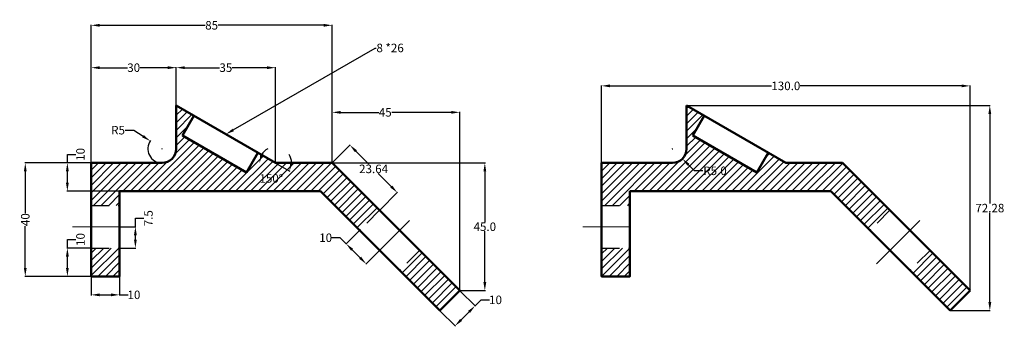
# Model space of a CAD drawing. Units: millimetres. Extents: x -10 to 337, y -40 to 68.
import ezdxf
from ezdxf import colors
from ezdxf.entities.mleader import LeaderData, LeaderLine
from ezdxf.math import Vec2, Vec3

# ---------------------------------------------------------------- set-up
doc = ezdxf.new("R2010")
doc.units = ezdxf.units.MM
doc.header["$MEASUREMENT"] = 0
doc.linetypes.add('CENTER', pattern=[50.8, 31.75, -6.35, 6.35, -6.35])
doc.linetypes.add('HIDDEN', pattern=[9.525, 6.35, -3.175])
for name, color, linetype, lineweight in [('M-CNTR', 1, 'CENTER', 18), ('M-DIMS', 3, 'Continuous', 25), ('M-HATC', 8, 'Continuous', 18), ('M-HIDN', 8, 'HIDDEN', 25), ('M-OUTL', 7, 'Continuous', 50)]:
    doc.layers.add(name, color=color, linetype=linetype, lineweight=lineweight)
doc.styles.get("Standard").update_dxf_attribs({"font": 'arial.ttf'})
doc.dimstyles.get("Standard").update_dxf_attribs({"dimtxt": 3, "dimasz": 3, "dimexe": 0.18, "dimexo": 0.0625, "dimgap": 0.09, "dimtad": 0, "dimtih": 1, "dimtoh": 1, "dimdec": 1, "dimdsep": 46, "dimtxsty": 'Standard', "dimcen": 0.09, "dimadec": 0, "dimazin": 0, "dimtfac": 1, "dimtdec": 1, "dimtofl": 0, "dimtmove": 0, "dimatfit": 3, "dimfxl": 1, "dimtolj": 1, "dimtzin": 0, "dimarcsym": 0})

# ---------------------------------------------------------------- blocks, each defined once
blk = doc.blocks.new('*D1')
at = {"layer": 'Defpoints', "color": 0, "transparency": 16777216}
for p in [(144.86, -27.53), (137.79, -34.6), (150.26, -32.93)]:
    blk.add_point(p, dxfattribs=at)
at = {"layer": 'M-DIMS', "color": 0, "lineweight": -2, "transparency": 16777216}
for p, q in [((144.9, -27.57), (150.39, -33.06)), ((150.26, -32.93), (152.39, -30.81)), ((152.39, -30.81), (155.39, -30.81)), ((137.83, -34.64), (143.32, -40.13)), ((145.32, -37.88), (148.14, -35.06))]:
    blk.add_line(p, q, dxfattribs=at)
at = {"layer": 'M-DIMS', "color": 0, "transparency": 16777216}
for points in [[(147.79, -34.7), (148.5, -35.41), (150.26, -32.93)], [(144.96, -37.53), (145.67, -38.24), (143.19, -40)]]:
    blk.add_solid(points, dxfattribs=at)
at = {"layer": 'M-DIMS', "color": 0, "transparency": 16777216, "insert": (157.48, -30.81), "char_height": 3, "attachment_point": 5}
blk.add_mtext('\\A1;10', dxfattribs=at)
blk = doc.blocks.new('*D2')
at = {"layer": 'Defpoints', "color": 0, "transparency": 16777216}
for p in [(144.86, 35.3), (99.86, 17.47), (144.86, -27.53)]:
    blk.add_point(p, dxfattribs=at)
at = {"layer": 'M-DIMS', "color": 0, "lineweight": -2, "transparency": 16777216}
for p, q in [((99.86, 17.53), (99.86, 35.48)), ((102.86, 35.3), (116.27, 35.3)), ((141.86, 35.3), (120.89, 35.3)), ((144.86, -27.47), (144.86, 35.48))]:
    blk.add_line(p, q, dxfattribs=at)
at = {"layer": 'M-DIMS', "color": 0, "transparency": 16777216}
for points in [[(102.86, 35.8), (102.86, 34.8), (99.86, 35.3)], [(141.86, 35.8), (141.86, 34.8), (144.86, 35.3)]]:
    blk.add_solid(points, dxfattribs=at)
at = {"layer": 'M-DIMS', "color": 0, "transparency": 16777216, "insert": (118.58, 35.3), "char_height": 3, "attachment_point": 5}
blk.add_mtext('\\A1;45', dxfattribs=at)
blk = doc.blocks.new('*D3')
at = {"layer": 'Defpoints', "color": 0, "transparency": 16777216}
for p in [(29.39, 46.61), (14.86, 17.47), (79.86, 17.47), (99.86, 17.47), (76.21, 13.13)]:
    blk.add_point(p, dxfattribs=at)
at = {"layer": 'M-DIMS', "color": 0, "lineweight": -2, "transparency": 16777216}
blk.add_line((79.91, 17.44), (84.93, 14.55), dxfattribs=at)
for start, end in [(118.6551, 149.3276), (0.6724, 31.3449)]:
    blk.add_arc((79.86, 17.47), 5.67, start, end, dxfattribs=at)
at = {"layer": 'M-DIMS', "color": 0, "transparency": 16777216}
for points in [[(75.46, 20.23), (74.5, 20.5), (74.19, 17.47)], [(86.01, 17.41), (85.05, 17.67), (84.77, 14.64)]]:
    blk.add_solid(points, dxfattribs=at)
at = {"layer": 'M-DIMS', "color": 0, "transparency": 16777216, "insert": (78.39, 11.99), "char_height": 3, "attachment_point": 5}
blk.add_mtext('\\A1;150°', dxfattribs=at)
blk = doc.blocks.new('*D4')
at = {"layer": 'Defpoints', "color": 0, "transparency": 16777216}
for p in [(109.5, -6.31), (104.78, -11.03), (116.57, -13.39)]:
    blk.add_point(p, dxfattribs=at)
at = {"layer": 'M-DIMS', "color": 0, "lineweight": -2, "transparency": 16777216}
for p, q in [((109.46, -6.36), (104.66, -11.16)), ((102.66, -8.91), (99.66, -8.91)), ((104.78, -11.03), (102.66, -8.91)), ((109.73, -15.98), (106.9, -13.16)), ((116.53, -13.43), (111.73, -18.23))]:
    blk.add_line(p, q, dxfattribs=at)
at = {"layer": 'M-DIMS', "color": 0, "transparency": 16777216}
for points in [[(107.26, -12.8), (106.55, -13.51), (104.78, -11.03)], [(110.09, -15.63), (109.38, -16.34), (111.85, -18.11)]]:
    blk.add_solid(points, dxfattribs=at)
at = {"layer": 'M-DIMS', "color": 0, "transparency": 16777216, "insert": (97.57, -8.91), "char_height": 3, "attachment_point": 5}
blk.add_mtext('\\A1;10', dxfattribs=at)
blk = doc.blocks.new('*D5')
at = {"layer": 'Defpoints', "color": 0, "transparency": 16777216}
for p in [(99.86, 65.99), (14.86, 17.47), (99.86, 17.47)]:
    blk.add_point(p, dxfattribs=at)
at = {"layer": 'M-DIMS', "color": 0, "lineweight": -2, "transparency": 16777216}
for p, q in [((14.86, 17.53), (14.86, 66.17)), ((17.86, 65.99), (55.11, 65.99)), ((96.86, 65.99), (59.61, 65.99)), ((99.86, 17.53), (99.86, 66.17))]:
    blk.add_line(p, q, dxfattribs=at)
at = {"layer": 'M-DIMS', "color": 0, "transparency": 16777216}
for points in [[(17.86, 66.49), (17.86, 65.49), (14.86, 65.99)], [(96.86, 66.49), (96.86, 65.49), (99.86, 65.99)]]:
    blk.add_solid(points, dxfattribs=at)
at = {"layer": 'M-DIMS', "color": 0, "transparency": 16777216, "insert": (57.36, 65.99), "char_height": 3, "attachment_point": 5}
blk.add_mtext('\\A1;85', dxfattribs=at)
blk = doc.blocks.new('*D6')
at = {"layer": 'Defpoints', "color": 0, "transparency": 16777216}
for p in [(44.86, 51.05), (44.86, 37.68), (14.86, 17.47)]:
    blk.add_point(p, dxfattribs=at)
at = {"layer": 'M-DIMS', "color": 0, "lineweight": -2, "transparency": 16777216}
for p, q in [((14.86, 17.53), (14.86, 51.23)), ((17.86, 51.05), (27.63, 51.05)), ((41.86, 51.05), (32.09, 51.05)), ((44.86, 37.74), (44.86, 51.23))]:
    blk.add_line(p, q, dxfattribs=at)
at = {"layer": 'M-DIMS', "color": 0, "transparency": 16777216}
for points in [[(17.86, 51.55), (17.86, 50.55), (14.86, 51.05)], [(41.86, 51.55), (41.86, 50.55), (44.86, 51.05)]]:
    blk.add_solid(points, dxfattribs=at)
at = {"layer": 'M-DIMS', "color": 0, "transparency": 16777216, "insert": (29.86, 51.05), "char_height": 3, "attachment_point": 5}
blk.add_mtext('\\A1;30', dxfattribs=at)
blk = doc.blocks.new('*D7')
at = {"layer": 'Defpoints', "color": 0, "transparency": 16777216}
for p in [(79.86, 51.05), (44.86, 37.68), (79.86, 17.47)]:
    blk.add_point(p, dxfattribs=at)
at = {"layer": 'M-DIMS', "color": 0, "lineweight": -2, "transparency": 16777216}
for p, q in [((44.86, 37.74), (44.86, 51.23)), ((47.86, 51.05), (60.11, 51.05)), ((76.86, 51.05), (64.61, 51.05)), ((79.86, 17.53), (79.86, 51.23))]:
    blk.add_line(p, q, dxfattribs=at)
at = {"layer": 'M-DIMS', "color": 0, "transparency": 16777216}
for points in [[(47.86, 51.55), (47.86, 50.55), (44.86, 51.05)], [(76.86, 51.55), (76.86, 50.55), (79.86, 51.05)]]:
    blk.add_solid(points, dxfattribs=at)
at = {"layer": 'M-DIMS', "color": 0, "transparency": 16777216, "insert": (62.36, 51.05), "char_height": 3, "attachment_point": 5}
blk.add_mtext('\\A1;35', dxfattribs=at)
blk = doc.blocks.new('*D8')
at = {"layer": 'Defpoints', "color": 0, "transparency": 16777216}
for p in [(35.68, 25.21), (39.86, 22.47)]:
    blk.add_point(p, dxfattribs=at)
at = {"layer": 'M-DIMS', "color": 0, "lineweight": -2, "transparency": 16777216}
for p, q in [((26.86, 29.02), (29.86, 29.02)), ((29.86, 29.02), (33.17, 26.86)), ((39.77, 22.47), (39.95, 22.47)), ((39.86, 22.38), (39.86, 22.56))]:
    blk.add_line(p, q, dxfattribs=at)
blk.add_arc((39.86, 22.47), 5, 144.7166, 269.2838, dxfattribs=at)
at = {"layer": 'M-DIMS', "color": 0, "transparency": 16777216}
blk.add_solid([(33.44, 27.27), (32.89, 26.44), (35.68, 25.21)], dxfattribs=at)
at = {"layer": 'M-DIMS', "color": 0, "transparency": 16777216, "insert": (24.34, 29.02), "char_height": 3, "attachment_point": 5}
blk.add_mtext('\\A1;R5', dxfattribs=at)
blk = doc.blocks.new('*D9')
at = {"layer": 'Defpoints', "color": 0, "transparency": 16777216}
for p in [(14.86, -22.53), (24.86, -22.53), (24.86, -29.04)]:
    blk.add_point(p, dxfattribs=at)
at = {"layer": 'M-DIMS', "color": 0, "lineweight": -2, "transparency": 16777216}
for p, q in [((14.86, -22.59), (14.86, -29.22)), ((24.86, -22.59), (24.86, -29.22)), ((17.86, -29.04), (21.86, -29.04)), ((24.86, -29.04), (27.86, -29.04))]:
    blk.add_line(p, q, dxfattribs=at)
at = {"layer": 'M-DIMS', "color": 0, "transparency": 16777216}
for points in [[(17.86, -28.54), (17.86, -29.54), (14.86, -29.04)], [(21.86, -28.54), (21.86, -29.54), (24.86, -29.04)]]:
    blk.add_solid(points, dxfattribs=at)
at = {"layer": 'M-DIMS', "color": 0, "transparency": 16777216, "insert": (29.95, -29.04), "char_height": 3, "attachment_point": 5}
blk.add_mtext('\\A1;10', dxfattribs=at)
blk = doc.blocks.new('*D10')
at = {"layer": 'Defpoints', "color": 0, "transparency": 16777216}
for p in [(6.47, -12.53), (14.86, -12.53), (14.86, -22.53)]:
    blk.add_point(p, dxfattribs=at)
at = {"layer": 'M-DIMS', "color": 0, "lineweight": -2, "transparency": 16777216}
for p, q in [((6.47, -12.53), (6.47, -9.53)), ((6.47, -9.53), (9.47, -9.53)), ((14.8, -12.53), (6.29, -12.53)), ((6.47, -19.53), (6.47, -15.53)), ((14.8, -22.53), (6.29, -22.53))]:
    blk.add_line(p, q, dxfattribs=at)
at = {"layer": 'M-DIMS', "color": 0, "transparency": 16777216}
for points in [[(5.97, -15.53), (6.97, -15.53), (6.47, -12.53)], [(5.97, -19.53), (6.97, -19.53), (6.47, -22.53)]]:
    blk.add_solid(points, dxfattribs=at)
at = {"layer": 'M-DIMS', "color": 0, "transparency": 16777216, "insert": (11.09, -9.53), "char_height": 3, "attachment_point": 5, "rotation": 90}
blk.add_mtext('\\A1;10', dxfattribs=at)
blk = doc.blocks.new('*D11')
at = {"layer": 'Defpoints', "color": 0, "transparency": 16777216}
for p in [(24.86, -5.03), (30.45, -5.03), (24.86, -12.53)]:
    blk.add_point(p, dxfattribs=at)
at = {"layer": 'M-DIMS', "color": 0, "lineweight": -2, "transparency": 16777216}
for p, q in [((30.45, -5.03), (30.45, -2.03)), ((30.45, -2.03), (33.45, -2.03)), ((24.92, -5.03), (30.63, -5.03)), ((30.45, -9.53), (30.45, -8.03)), ((24.92, -12.53), (30.63, -12.53))]:
    blk.add_line(p, q, dxfattribs=at)
at = {"layer": 'M-DIMS', "color": 0, "transparency": 16777216}
for points in [[(29.95, -8.03), (30.95, -8.03), (30.45, -5.03)], [(29.95, -9.53), (30.95, -9.53), (30.45, -12.53)]]:
    blk.add_solid(points, dxfattribs=at)
at = {"layer": 'M-DIMS', "color": 0, "transparency": 16777216, "insert": (35.06, -2.03), "char_height": 3, "attachment_point": 5, "rotation": 90}
blk.add_mtext('\\A1;7.5', dxfattribs=at)
blk = doc.blocks.new('*D12')
at = {"layer": 'Defpoints', "color": 0, "transparency": 16777216}
for p in [(-8.38, 17.47), (14.86, 17.47), (14.86, -22.53)]:
    blk.add_point(p, dxfattribs=at)
at = {"layer": 'M-DIMS', "color": 0, "lineweight": -2, "transparency": 16777216}
for p, q in [((14.8, 17.47), (-8.56, 17.47)), ((-8.38, 14.47), (-8.38, -0.23)), ((-8.38, -19.53), (-8.38, -4.82)), ((14.8, -22.53), (-8.56, -22.53))]:
    blk.add_line(p, q, dxfattribs=at)
at = {"layer": 'M-DIMS', "color": 0, "transparency": 16777216}
for points in [[(-8.88, 14.47), (-7.88, 14.47), (-8.38, 17.47)], [(-8.88, -19.53), (-7.88, -19.53), (-8.38, -22.53)]]:
    blk.add_solid(points, dxfattribs=at)
at = {"layer": 'M-DIMS', "color": 0, "transparency": 16777216, "insert": (-8.38, -2.53), "char_height": 3, "attachment_point": 5, "rotation": 90}
blk.add_mtext('\\A1;40', dxfattribs=at)
blk = doc.blocks.new('*D13')
at = {"layer": 'Defpoints', "color": 0, "transparency": 16777216}
for p in [(6.46, 17.47), (14.86, 17.47), (24.86, 7.47)]:
    blk.add_point(p, dxfattribs=at)
at = {"layer": 'M-DIMS', "color": 0, "lineweight": -2, "transparency": 16777216}
for p, q in [((14.8, 17.47), (6.28, 17.47)), ((6.46, 17.47), (6.46, 20.47)), ((6.46, 20.47), (9.46, 20.47)), ((6.46, 10.47), (6.46, 14.47)), ((24.8, 7.47), (6.28, 7.47))]:
    blk.add_line(p, q, dxfattribs=at)
at = {"layer": 'M-DIMS', "color": 0, "transparency": 16777216}
for points in [[(5.96, 14.47), (6.96, 14.47), (6.46, 17.47)], [(5.96, 10.47), (6.96, 10.47), (6.46, 7.47)]]:
    blk.add_solid(points, dxfattribs=at)
at = {"layer": 'M-DIMS', "color": 0, "transparency": 16777216, "insert": (11.08, 20.47), "char_height": 3, "attachment_point": 5, "rotation": 90}
blk.add_mtext('\\A1;10', dxfattribs=at)
blk = doc.blocks.new('*D14')
at = {"layer": 'Defpoints', "color": 0, "transparency": 16777216}
for p in [(224.87, 37.68), (317.8, -34.6), (331.82, -34.6)]:
    blk.add_point(p, dxfattribs=at)
at = {"layer": 'M-DIMS', "color": 0, "lineweight": -2, "transparency": 16777216}
for p, q in [((224.93, 37.68), (332, 37.68)), ((331.82, 34.68), (331.82, 3.16)), ((331.82, -31.6), (331.82, -0.08)), ((317.86, -34.6), (332, -34.6))]:
    blk.add_line(p, q, dxfattribs=at)
at = {"layer": 'M-DIMS', "color": 0, "transparency": 16777216}
for points in [[(331.32, 34.68), (332.32, 34.68), (331.82, 37.68)], [(331.32, -31.6), (332.32, -31.6), (331.82, -34.6)]]:
    blk.add_solid(points, dxfattribs=at)
at = {"layer": 'M-DIMS', "color": 0, "transparency": 16777216, "insert": (331.82, 1.54), "char_height": 3, "attachment_point": 5}
blk.add_mtext('\\A1;72.28', dxfattribs=at)
blk = doc.blocks.new('*D15')
at = {"layer": 'Defpoints', "color": 0, "transparency": 16777216}
for p in [(324.87, 44.63), (194.87, 17.47), (324.87, -27.53)]:
    blk.add_point(p, dxfattribs=at)
at = {"layer": 'M-DIMS', "color": 0, "lineweight": -2, "transparency": 16777216}
for p, q in [((194.87, 17.53), (194.87, 44.81)), ((197.87, 44.63), (254.86, 44.63)), ((321.87, 44.63), (264.87, 44.63)), ((324.87, -27.47), (324.87, 44.81))]:
    blk.add_line(p, q, dxfattribs=at)
at = {"layer": 'M-DIMS', "color": 0, "transparency": 16777216}
for points in [[(197.87, 45.13), (197.87, 44.13), (194.87, 44.63)], [(321.87, 45.13), (321.87, 44.13), (324.87, 44.63)]]:
    blk.add_solid(points, dxfattribs=at)
at = {"layer": 'M-DIMS', "color": 0, "transparency": 16777216, "insert": (259.87, 44.63), "char_height": 3, "attachment_point": 5}
blk.add_mtext('\\A1;130.0', dxfattribs=at)
blk = doc.blocks.new('*D16')
at = {"layer": 'Defpoints', "color": 0, "transparency": 16777216}
for p in [(99.86, 17.47), (144.86, -27.53), (153.71, -27.53)]:
    blk.add_point(p, dxfattribs=at)
at = {"layer": 'M-DIMS', "color": 0, "lineweight": -2, "transparency": 16777216}
for p, q in [((99.92, 17.47), (153.89, 17.47)), ((153.71, 14.47), (153.71, -3.41)), ((153.71, -24.53), (153.71, -6.65)), ((144.92, -27.53), (153.89, -27.53))]:
    blk.add_line(p, q, dxfattribs=at)
at = {"layer": 'M-DIMS', "color": 0, "transparency": 16777216}
for points in [[(153.21, 14.47), (154.21, 14.47), (153.71, 17.47)], [(153.21, -24.53), (154.21, -24.53), (153.71, -27.53)]]:
    blk.add_solid(points, dxfattribs=at)
at = {"layer": 'M-DIMS', "color": 0, "transparency": 16777216, "insert": (153.71, -5.03), "char_height": 3, "attachment_point": 5}
blk.add_mtext('\\A1;45.0', dxfattribs=at)
blk = doc.blocks.new('*D17')
at = {"layer": 'Defpoints', "color": 0, "transparency": 16777216}
for p in [(99.86, 17.47), (122.83, 7.01), (116.57, 0.76)]:
    blk.add_point(p, dxfattribs=at)
at = {"layer": 'M-DIMS', "color": 0, "lineweight": -2, "transparency": 16777216}
for p, q in [((99.9, 17.52), (106.24, 23.86)), ((108.24, 21.61), (112.85, 17)), ((120.71, 9.14), (116.1, 13.75)), ((116.62, 0.8), (122.96, 7.14))]:
    blk.add_line(p, q, dxfattribs=at)
at = {"layer": 'M-DIMS', "color": 0, "transparency": 16777216}
for points in [[(108.59, 21.96), (107.88, 21.26), (106.12, 23.73)], [(121.06, 9.49), (120.36, 8.78), (122.83, 7.01)]]:
    blk.add_solid(points, dxfattribs=at)
at = {"layer": 'M-DIMS', "color": 0, "transparency": 16777216, "insert": (114.47, 15.37), "char_height": 3, "attachment_point": 5}
blk.add_mtext('\\A1;23.64', dxfattribs=at)
blk = doc.blocks.new('*D18')
at = {"layer": 'Defpoints', "color": 0, "transparency": 16777216}
for p in [(219.87, 22.47), (223.4, 18.94)]:
    blk.add_point(p, dxfattribs=at)
at = {"layer": 'M-DIMS', "color": 0, "lineweight": -2, "transparency": 16777216}
for p, q in [((219.78, 22.47), (219.96, 22.47)), ((219.87, 22.38), (219.87, 22.56)), ((227.65, 14.69), (225.52, 16.81)), ((230.65, 14.69), (227.65, 14.69))]:
    blk.add_line(p, q, dxfattribs=at)
at = {"layer": 'M-DIMS', "color": 0, "transparency": 16777216}
blk.add_solid([(225.88, 17.17), (225.17, 16.46), (223.4, 18.94)], dxfattribs=at)
at = {"layer": 'M-DIMS', "color": 0, "transparency": 16777216, "insert": (234.9, 14.69), "char_height": 3, "attachment_point": 5}
blk.add_mtext('\\A1;R5.0', dxfattribs=at)

msp = doc.modelspace()

# ---------------------------------------------------------------- hatches: boundary and pattern name
at = {"layer": 'M-HATC'}
h = msp.add_hatch(dxfattribs=at)
h.set_pattern_fill('ANSI31', color=256, scale=15)
h.paths.add_polyline_path([(24.859, -12.528), (14.859, -12.528), (14.859, -22.528), (24.859, -22.528)])
h.paths.add_polyline_path([(47.1, 27.148), (51.1, 34.076), (44.859, 37.68), (44.859, 22.472, -0.4142136), (39.859, 17.472), (14.859, 17.472), (14.859, 2.472), (24.859, 2.472), (24.859, 7.472), (95.717, 7.472), (109.503, -6.314), (116.575, 0.757), (99.859, 17.472), (79.859, 17.472), (73.617, 21.076), (69.617, 14.148)])
h.paths.add_polyline_path([(130.717, -13.386), (123.646, -20.457), (137.788, -34.599), (144.859, -27.528)])
h = msp.add_hatch(dxfattribs=at)
h.set_pattern_fill('ANSI31', color=256, scale=15)
h.paths.add_polyline_path([(204.869, -12.528), (194.869, -12.528), (194.869, -22.528), (204.869, -22.528)])
h.paths.add_polyline_path([(279.869, 17.472), (259.869, 17.472), (253.628, 21.076), (249.628, 14.148), (227.111, 27.148), (231.111, 34.076), (224.869, 37.68), (224.869, 22.472, -0.4142136), (219.869, 17.472), (194.869, 17.472), (194.869, 2.472), (204.869, 2.472), (204.869, 7.472), (275.727, 7.472), (289.514, -6.314), (296.585, 0.757)])
h.paths.add_polyline_path([(310.727, -13.386), (303.656, -20.457), (317.798, -34.599), (324.869, -27.528)])

# ---------------------------------------------------------------- linework, layer by layer
at = {"layer": 'M-CNTR'}
for p, q in [((127.172, -2.788), (111.867, -18.094)), ((307.183, -2.788), (291.877, -18.094)), ((8.272, -5.028), (24.859, -5.028)), ((188.283, -5.028), (204.869, -5.028))]:
    msp.add_line(p, q, dxfattribs=at)
at = {"layer": 'M-HIDN'}
for p, q in [((14.859, 2.472), (24.859, 2.472)), ((116.575, 0.757), (109.503, -6.314)), ((194.869, 2.472), (204.869, 2.472)), ((296.585, 0.757), (289.514, -6.314)), ((14.859, -12.528), (24.859, -12.528)), ((130.717, -13.386), (123.646, -20.457)), ((194.869, -12.528), (204.869, -12.528)), ((310.727, -13.386), (303.656, -20.457))]:
    msp.add_line(p, q, dxfattribs=at)
at = {"layer": 'M-OUTL'}
for p, q in [((44.859, 22.472), (44.859, 37.68)), ((79.859, 17.472), (44.859, 37.68)), ((224.869, 22.472), (224.869, 37.68)), ((259.869, 17.472), (224.869, 37.68)), ((51.1, 34.076), (47.1, 27.148)), ((231.111, 34.076), (227.111, 27.148)), ((47.1, 27.148), (69.617, 14.148)), ((227.111, 27.148), (249.628, 14.148)), ((73.617, 21.076), (69.617, 14.148)), ((253.628, 21.076), (249.628, 14.148)), ((14.859, 17.472), (39.859, 17.472)), ((99.859, 17.472), (144.859, -27.528)), ((194.869, 17.472), (219.869, 17.472)), ((279.869, 17.472), (324.869, -27.528)), ((95.717, 7.472), (137.788, -34.599)), ((275.727, 7.472), (317.798, -34.599)), ((14.859, -22.528), (14.859, -12.528)), ((194.869, -22.528), (194.869, -12.528)), ((144.859, -27.528), (137.788, -34.599)), ((144.859, -27.528), (139.859, -32.528)), ((324.869, -27.528), (317.798, -34.599)), ((324.869, -27.528), (319.869, -32.528))]:
    msp.add_line(p, q, dxfattribs=at)
for points in [[(14.859, 7.472), (14.859, 17.472), (39.859, 17.472)], [(24.859, 7.472), (24.859, -22.528), (14.859, -22.528), (14.859, 17.472), (24.859, 17.472)], [(79.859, 17.472), (99.859, 17.472)], [(194.869, 7.472), (194.869, 17.472), (219.869, 17.472)], [(204.869, 7.472), (204.869, -22.528), (194.869, -22.528), (194.869, 17.472), (204.869, 17.472)], [(259.869, 17.472), (279.869, 17.472)], [(95.717, 7.472), (24.859, 7.472)], [(275.727, 7.472), (204.869, 7.472)]]:
    msp.add_lwpolyline(points, dxfattribs=at)
for centre in [(39.859, 22.472), (219.869, 22.472)]:
    msp.add_arc(centre, 5, 270, 0, dxfattribs=at)

# ---------------------------------------------------------------- dimensions: what is measured, and where the dimension line sits
at = {"layer": 'M-DIMS', "transparency": 33554610}
for base, p1, p2, picture, middle in [((99.859, 65.995), (14.859, 17.472), (99.859, 17.472), '*D5', (57.359, 65.995)), ((44.859, 51.053), (14.859, 17.472), (44.859, 37.68), '*D6', (29.859, 51.053)), ((79.859, 51.053), (44.859, 37.68), (79.859, 17.472), '*D7', (62.359, 51.053)), ((24.859, -29.041), (14.859, -22.528), (24.859, -22.528), '*D9', (29.951, -29.041))]:
    dim = msp.add_linear_dim(base=base, p1=p1, p2=p2, dimstyle='Standard', override={"dimclrd": 0, "dimclre": 0, "dimclrt": 0}, dxfattribs=at)
    dim.commit()
    dim.dimension.update_dxf_attribs({"geometry": picture, "text_midpoint": middle})
dim = msp.add_angular_dim_2l(base=(76.213, 13.128), line1=((14.859, 17.472), (99.859, 17.472)), line2=((79.859, 17.472), (29.387, 46.612)), dimstyle='Standard', override={"dimclrd": 0, "dimclre": 0, "dimclrt": 0}, dxfattribs=at)
dim.commit()
dim.dimension.update_dxf_attribs({"geometry": '*D3', "text_midpoint": (78.391, 11.994)})
at = {"layer": 'M-DIMS'}
dim = msp.add_linear_dim(base=(324.869, 44.63), p1=(194.869, 17.472), p2=(324.869, -27.528), dimstyle='Standard', override={"dimdec": 1, "dimlfac": 1, "dimrnd": 0, "dimzin": 0, "dimdsep": 46, "dimlunit": 2}, dxfattribs=at)
dim.commit()
dim.dimension.update_dxf_attribs({"geometry": '*D15', "text_midpoint": (259.869, 44.63)})
at = {"layer": 'M-DIMS', "transparency": 33554610}
dim = msp.add_linear_dim(base=(144.859, 35.304), p1=(99.859, 17.472), p2=(144.859, -27.528), dimstyle='Standard', override={"dimclrd": 0, "dimclre": 0, "dimclrt": 0}, dxfattribs=at)
dim.commit()
dim.dimension.update_dxf_attribs({"geometry": '*D2', "text_midpoint": (118.578, 35.304), "dimtype": 160})
at = {"layer": 'M-DIMS'}
for base, p1, p2, angle, override, picture, middle in [((331.819, -34.599), (224.869, 37.68), (317.798, -34.599), 90, {"dimdec": 2, "dimlfac": 1, "dimrnd": 0, "dimzin": 0, "dimdsep": 46, "dimlunit": 2}, '*D14', (331.819, 1.54)), ((122.832, 7.014), (99.859, 17.472), (116.575, 0.757), 315, {"dimdec": 2, "dimlfac": 1, "dimrnd": 0, "dimzin": 0, "dimdsep": 46, "dimlunit": 2}, '*D17', (114.475, 15.372)), ((153.709, -27.528), (99.859, 17.472), (144.859, -27.528), 90, {"dimdec": 1, "dimlfac": 1, "dimrnd": 0, "dimzin": 0, "dimdsep": 46, "dimlunit": 2}, '*D16', (153.709, -5.028))]:
    dim = msp.add_linear_dim(base=base, p1=p1, p2=p2, angle=angle, dimstyle='Standard', override=override, dxfattribs=at)
    dim.commit()
    dim.dimension.update_dxf_attribs({"geometry": picture, "text_midpoint": middle})
at = {"layer": 'M-DIMS', "transparency": 33554610}
dim = msp.add_radius_dim(center=(39.859, 22.472), mpoint=(35.676, 25.212), dimstyle='Standard', override={"dimclrd": 0, "dimclre": 0, "dimclrt": 0}, dxfattribs=at)
dim.commit()
dim.dimension.update_dxf_attribs({"geometry": '*D8', "text_midpoint": (24.34, 29.02), "dimtype": 164})
for base, p1, p2, picture, middle in [((6.461, 17.472), (24.859, 7.472), (14.859, 17.472), '*D13', (11.083, 20.472)), ((-8.384, 17.472), (14.859, -22.528), (14.859, 17.472), '*D12', (-8.384, -2.528)), ((30.446, -5.028), (24.859, -12.528), (24.859, -5.028), '*D11', (35.062, -2.028)), ((6.466, -12.528), (14.859, -22.528), (14.859, -12.528), '*D10', (11.088, -9.528))]:
    dim = msp.add_linear_dim(base=base, p1=p1, p2=p2, angle=90, dimstyle='Standard', override={"dimclrd": 0, "dimclre": 0, "dimclrt": 0}, dxfattribs=at)
    dim.commit()
    dim.dimension.update_dxf_attribs({"geometry": picture, "text_midpoint": middle, "text_rotation": 90})
at = {"layer": 'M-DIMS'}
dim = msp.add_radius_dim(center=(219.869, 22.472), mpoint=(223.404, 18.936), dimstyle='Standard', override={"dimdec": 1, "dimlfac": 1, "dimrnd": 0, "dimzin": 0, "dimdsep": 46, "dimlunit": 2}, dxfattribs=at)
dim.commit()
dim.dimension.update_dxf_attribs({"geometry": '*D18', "text_midpoint": (234.897, 14.692)})
at = {"layer": 'M-DIMS', "transparency": 33554610}
for p1, p2, distance, picture, middle in [((116.575, -13.386), (109.503, -6.314), 6.675, '*D4', (97.569, -8.913)), ((137.788, -34.599), (144.859, -27.528), -7.645, '*D1', (157.479, -30.812))]:
    dim = msp.add_aligned_dim(p1=p1, p2=p2, distance=distance, dimstyle='Standard', override={"dimclrd": 0, "dimclre": 0, "dimclrt": 0}, dxfattribs=at)
    dim.commit()
    dim.dimension.update_dxf_attribs({"geometry": picture, "text_midpoint": middle})

# ---------------------------------------------------------------- leaders
ml = msp.add_multileader_mtext('Standard', dxfattribs=at)
ml.set_content('8 *26', color=256)
ml.set_leader_properties()
ml.build(insert=Vec2(0, 0))
ml.multileader.update_dxf_attribs({"dogleg_length": 0.36, "arrow_head_size": 3})
ctx = ml.context
ctx.base_point, ctx.char_height, ctx.arrow_head_size, ctx.landing_gap_size, ctx.plane_origin = Vec3(115.388, 57.984), 3, 3, 0.09, Vec3(62.359, 27.576)
notes = []
notes.append((ctx, [(0, (1, 1, 0), (115.028, 57.984), (1, 0), 0.36, [(0, [(62.359, 27.576)], 0, [])])]))
ctx.mtext.insert, ctx.mtext.flow_direction = Vec3(115.478, 59.51), 5
for ctx, leaders in notes:
    for number, flags, end, landing, length, lines in leaders:
        leader = LeaderData()
        leader.index, (leader.has_last_leader_line, leader.has_dogleg_vector, leader.attachment_direction) = number, flags
        leader.last_leader_point, leader.dogleg_vector, leader.dogleg_length = Vec3(end), Vec3(landing), length
        for number, points, colour, breaks in lines:
            line = LeaderLine()
            line.index, line.vertices, line.color, line.breaks = number, Vec3.list(points), colors.encode_raw_color(colour), breaks
            leader.lines.append(line)
        ctx.leaders.append(leader)

doc.saveas('drawing.dxf')
